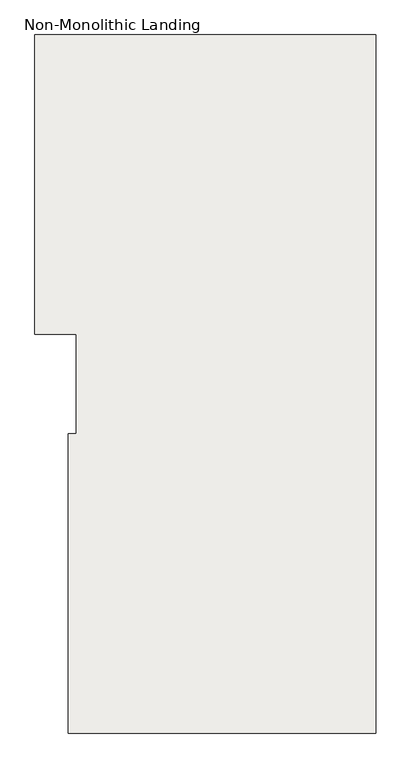
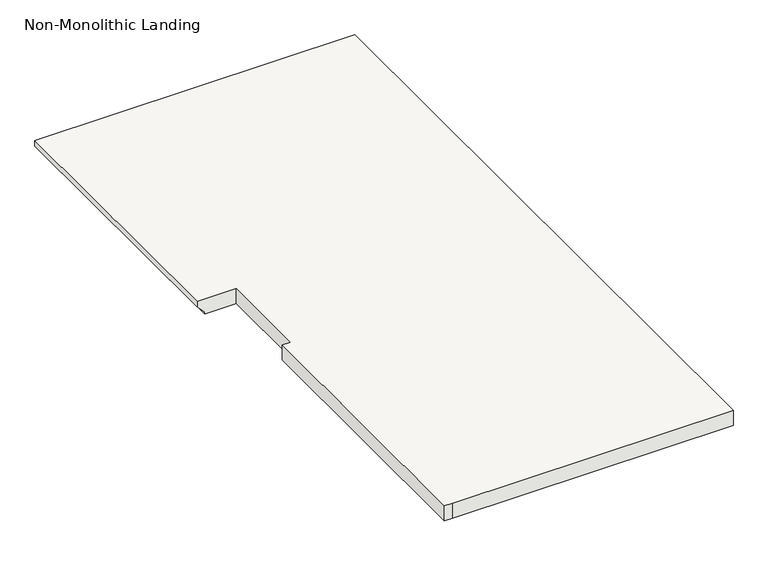
"""IFC4 building model written with IfcOpenShell, lengths in millimetres: slab geometry, Non-Monolithic Landing."""

from ifc_helpers import new_model, si_unit, origin, place, context, project, spatial, faceted_brep, source, transform, mapped, element, save


def non_monolithic_landing_52da1c58(model_context):
    return source(origin(), model_context, "Body", "Brep", [
        faceted_brep([(551.235938, 2339.7857363, 4688.4166667), (551.235938, 2339.7857363, 4707.4666667), (551.235938, 3254.1857363, 4707.4666667), (551.235938, 3254.1857363, 4688.4166667), (576.635938, 2339.7857363, 4663.0166667), (576.635938, 3254.1857363, 4663.0166667), (678.235938, 2339.7857363, 4707.4666667), (678.235938, 2034.9857363, 4707.4666667), (652.835938, 2034.9857363, 4707.4666667), (652.835938, 1120.5857363, 4707.4666667), (678.235938, 1120.5857363, 4707.4666667), (1592.635938, 1120.5857363, 4707.4666667), (1592.635938, 3254.1857363, 4707.4666667), (576.635938, 2339.7857363, 4656.6666667), (576.635938, 3254.1857363, 4656.6666667), (1592.635938, 3254.1857363, 4656.6666667), (1592.635938, 1120.5857363, 4656.6666667), (678.235938, 1120.5857363, 4656.6666667), (652.835938, 1120.5857363, 4656.6666667), (652.835938, 2034.9857363, 4656.6666667), (678.235938, 2034.9857363, 4656.6666667), (678.235938, 2339.7857363, 4656.6666667)], [[[0, 1, 2, 3]], [[4, 0, 3, 5]], [[6, 7, 8, 9, 10, 11, 12, 2, 1]], [[13, 14, 15, 16, 17, 18, 19, 20, 21]], [[14, 13, 4, 5]], [[6, 1, 0, 4, 13, 21]], [[7, 6, 21, 20]], [[8, 7, 20, 19]], [[9, 8, 19, 18]], [[10, 9, 18, 17]], [[11, 10, 17, 16]], [[12, 11, 16, 15]], [[2, 12, 15, 14, 5, 3]]]),
    ])


if __name__ == "__main__":
    model = new_model("IFC4")
    model_context = context("Model", 3, world=origin())
    ifc_project = project(units=[si_unit("LENGTHUNIT", "METRE", prefix="MILLI")], contexts=[model_context])
    site = spatial("IfcSite", under=ifc_project)
    building = spatial("IfcBuilding", under=site)
    placement = place(None, origin())
    non_monolithic_landing_shape = non_monolithic_landing_52da1c58(model_context)
    element("IfcSlab", 1, ObjectType="Non-Monolithic Landing", at=placement, inside=building, context=model_context, shape_type="MappedRepresentation", body=[
        mapped(non_monolithic_landing_shape, transform((0.0, 0.0, 0.0), x_axis=(1.0, 0.0, 0.0), y_axis=(0.0, 1.0, 0.0), z_axis=(0.0, 0.0, 1.0))),
    ])
    save(model, "model.ifc")

# Revit data of these elements
# Element 1 (IfcSlab, "Non-Monolithic Landing")
#   Materials on its faces: "BURGUNDY COLOUR"
# Materials
#   "BURGUNDY COLOUR": class "Generic", colour RGB 120 120 120, transparency 0, Cost = 0
